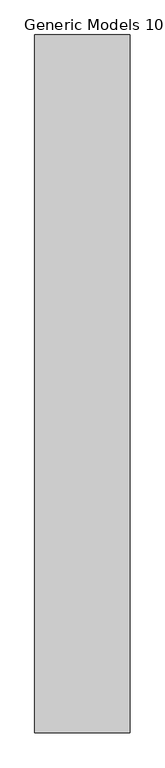
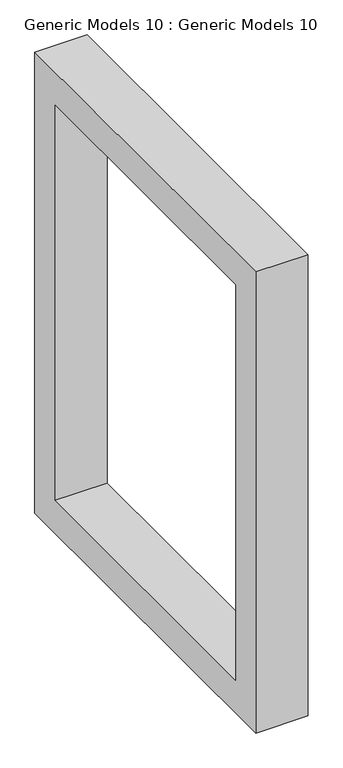
"""IFC4 building model written with IfcOpenShell, lengths in millimetres: proxy geometry, Generic Models 10 : Generic Models 10."""

from ifc_helpers import new_model, si_unit, frame, origin, place, context, project, spatial, polyline, outline, extrude, source, transform, mapped, element, save


def generic_models_10_generic_models_10_8dbd4941(model_context):
    return source(origin(), model_context, "Body", "SweptSolid", [
        extrude(outline(polyline([(4025.9641252, 9353.8433359), (5143.5641252, 9353.8433359), (5143.5641252, 7931.4433359), (4025.9641252, 7931.4433359), (4025.9641252, 9353.8433359)]), holes=[polyline([(4127.5641252, 9252.2433359), (4127.5641252, 8033.0433359), (5041.9641252, 8033.0433359), (5041.9641252, 9252.2433359), (4127.5641252, 9252.2433359)])]), frame((-6249.8280307, 0.0, 0.0), z_axis=(1.0, 0.0, 0.0), x_axis=(0.0, 1.0, 0.0)), (0.0, 0.0, 1.0), 152.4),
    ])


if __name__ == "__main__":
    model = new_model("IFC4")
    model_context = context("Model", 3, world=origin())
    ifc_project = project(units=[si_unit("LENGTHUNIT", "METRE", prefix="MILLI")], contexts=[model_context])
    site = spatial("IfcSite", under=ifc_project)
    building = spatial("IfcBuilding", under=site)
    placement = place(None, origin())
    generic_models_10_generic_models_10_shape = generic_models_10_generic_models_10_8dbd4941(model_context)
    element("IfcBuildingElementProxy", 1, Name="Generic Models 10 : Generic Models 10", ObjectType="Generic Models 10 : Generic Models 10", at=placement, inside=building, context=model_context, shape_type="MappedRepresentation", body=[
        mapped(generic_models_10_generic_models_10_shape, transform((0.0, 0.0, 0.0), x_axis=(1.0, 0.0, 0.0), y_axis=(0.0, 1.0, 0.0), z_axis=(0.0, 0.0, 1.0))),
    ])
    save(model, "model.ifc")

# Revit data of these elements
# Element 1 (IfcBuildingElementProxy, "Generic Models 10 : Generic Models 10")
#   Materials on its faces: "chocolate brown"
# Materials
#   "chocolate brown": class "Generic", colour RGB 120 120 120, transparency 0, Cost = 0
